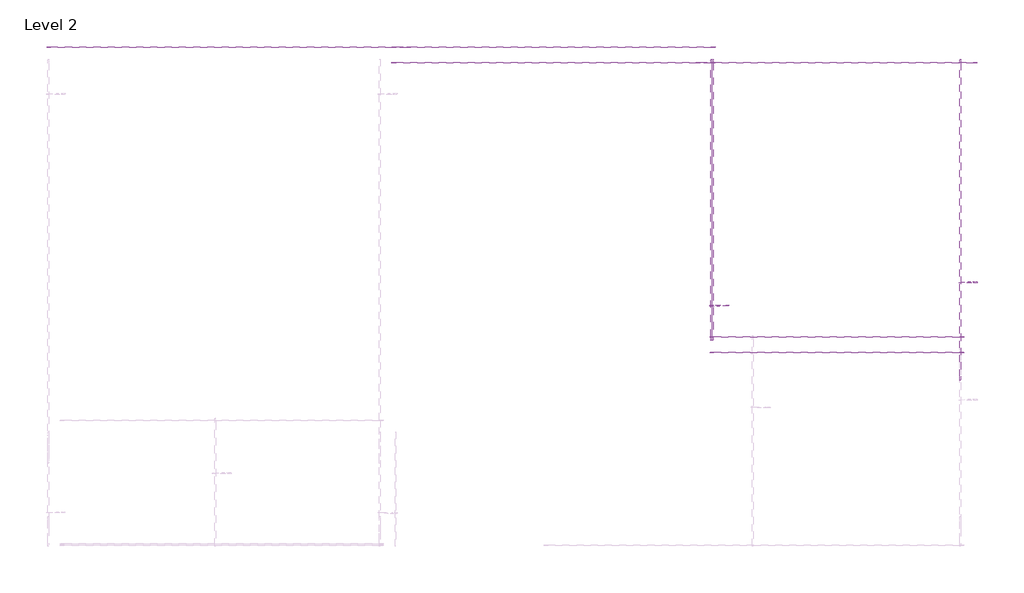
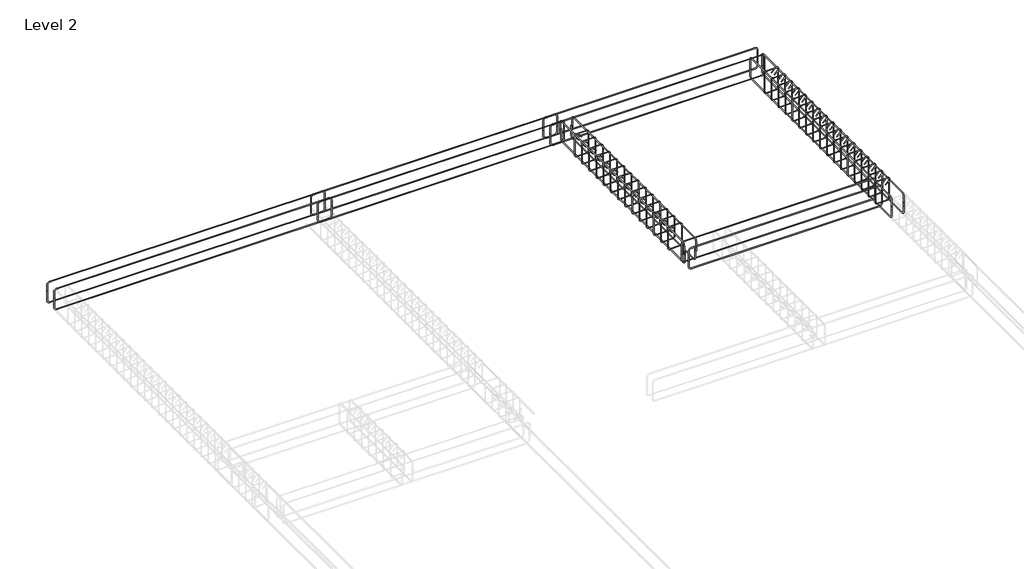
# One storey, part 5 of 5: 14 reinforcing bars.
"""IFC4 building model written with IfcOpenShell, lengths in millimetres."""

from ifc_helpers import new_model, si_unit, point, frame, origin, place, context, project, spatial, polyline, circle_curve, trimmed, segment, composite_curve, source, transform, mapped, element, save
from ifc_brep_helpers import swept_disk

model = new_model("IFC4")

# Units and contexts
model_context = context("Model", 3, world=origin())
ifc_project = project(units=[si_unit("LENGTHUNIT", "METRE", prefix="MILLI")], contexts=[model_context])

# Site, building, storey
site = spatial("IfcSite", under=ifc_project)
building = spatial("IfcBuilding", under=site)
storey = spatial("IfcBuildingStorey", under=building, Name="Level 2", Elevation=3048.0)

# Reinforcing bars
placement = place(None, origin())
reinforcing_bar_shape = source(origin(), model_context, "Body", "SolidModel", [
    swept_disk(composite_curve([segment(polyline([(-11033.7905379, 8472.592544, 5892.9032081), (-11033.7905379, 8472.592544, 5740.5032081)]), True, "CONTINUOUS"), segment(trimmed(circle_curve(frame((-11077.8595379, 8472.592544, 5740.5032081), z_axis=(0.0, 1.0, 0.0), x_axis=(44.068999999999505, 0.0, 0.0)), 44.069), [point((-11033.7905379, 8472.592544, 5740.5032081))], [point((-11077.8595379, 8472.592544, 5696.4342081))], True, "CARTESIAN"), True, "CONTINUOUS"), segment(polyline([(-11077.8595379, 8472.592544, 5696.4342081), (-15371.4835379, 8472.592544, 5696.4342081)]), True, "CONTINUOUS"), segment(trimmed(circle_curve(frame((-15371.4835379, 8472.592544, 5740.5032081), z_axis=(0.0, 1.0, 0.0), x_axis=(0.0, 0.0, -44.068999999999505)), 44.069), [point((-15371.4835379, 8472.592544, 5696.4342081))], [point((-15415.5525379, 8472.592544, 5740.5032081))], True, "CARTESIAN"), True, "CONTINUOUS"), segment(polyline([(-15415.5525379, 8472.592544, 5740.5032081), (-15415.5525379, 8472.592544, 5892.9032081)]), True, "CONTINUOUS")], self_intersect=False), 5.969),
])
element("IfcReinforcingBar", 1, at=placement, inside=storey, context=model_context, shape_type="MappedRepresentation", body=[
    mapped(reinforcing_bar_shape, transform((0.0, 0.0, 0.0), x_axis=(1.0, 0.0, 0.0), y_axis=(0.0, 1.0, 0.0), z_axis=(0.0, 0.0, 1.0))),
    mapped(reinforcing_bar_shape, transform((0.0, -189.5315837, 0.0), x_axis=(1.0, 0.0, 0.0), y_axis=(0.0, 1.0, 0.0), z_axis=(0.0, 0.0, 1.0))),
])
reinforcing_bar_2_shape = source(origin(), model_context, "Body", "SolidModel", [
    swept_disk(composite_curve([segment(polyline([(-15415.5525379, 8472.592544, 5841.8967919), (-15415.5525379, 8472.592544, 5994.2967919)]), True, "CONTINUOUS"), segment(trimmed(circle_curve(frame((-15371.4835379, 8472.592544, 5994.2967919), z_axis=(0.0, 1.0, 0.0), x_axis=(-44.068999999999505, 0.0, 0.0)), 44.069), [point((-15415.5525379, 8472.592544, 5994.2967919))], [point((-15371.4835379, 8472.592544, 6038.3657919))], True, "CARTESIAN"), True, "CONTINUOUS"), segment(polyline([(-15371.4835379, 8472.592544, 6038.3657919), (-11077.8595379, 8472.592544, 6038.3657919)]), True, "CONTINUOUS"), segment(trimmed(circle_curve(frame((-11077.8595379, 8472.592544, 5994.2967919), z_axis=(0.0, 1.0, 0.0), x_axis=(0.0, 0.0, 44.068999999999505)), 44.069), [point((-11077.8595379, 8472.592544, 6038.3657919))], [point((-11033.7905379, 8472.592544, 5994.2967919))], True, "CARTESIAN"), True, "CONTINUOUS"), segment(polyline([(-11033.7905379, 8472.592544, 5994.2967919), (-11033.7905379, 8472.592544, 5841.8967919)]), True, "CONTINUOUS")], self_intersect=False), 5.969),
])
element("IfcReinforcingBar", 2, at=placement, inside=storey, context=model_context, shape_type="MappedRepresentation", body=[
    mapped(reinforcing_bar_2_shape, transform((0.0, 0.0, 0.0), x_axis=(1.0, 0.0, 0.0), y_axis=(0.0, 1.0, 0.0), z_axis=(0.0, 0.0, 1.0))),
    mapped(reinforcing_bar_2_shape, transform((0.0, -189.5315837, 0.0), x_axis=(1.0, 0.0, 0.0), y_axis=(0.0, 1.0, 0.0), z_axis=(0.0, 0.0, 1.0))),
])
reinforcing_bar_3_shape = source(origin(), model_context, "Body", "SolidModel", [
    swept_disk(composite_curve([segment(polyline([(-11250.4525379, 8472.592544, 5841.8967919), (-11250.4525379, 8472.592544, 5994.2967919)]), True, "CONTINUOUS"), segment(trimmed(circle_curve(frame((-11206.3835379, 8472.592544, 5994.2967919), z_axis=(0.0, 1.0, 0.0), x_axis=(-44.069000000001324, 0.0, 0.0)), 44.069), [point((-11250.4525379, 8472.592544, 5994.2967919))], [point((-11206.3835379, 8472.592544, 6038.3657919))], True, "CARTESIAN"), True, "CONTINUOUS"), segment(polyline([(-11206.3835379, 8472.592544, 6038.3657919), (-7408.0595379, 8472.592544, 6038.3657919)]), True, "CONTINUOUS"), segment(trimmed(circle_curve(frame((-7408.0595379, 8472.592544, 5994.2967919), z_axis=(0.0, 1.0, 0.0), x_axis=(0.0, 0.0, 44.068999999999505)), 44.069), [point((-7408.0595379, 8472.592544, 6038.3657919))], [point((-7363.9905379, 8472.592544, 5994.2967919))], True, "CARTESIAN"), True, "CONTINUOUS"), segment(polyline([(-7363.9905379, 8472.592544, 5994.2967919), (-7363.9905379, 8472.592544, 5841.8967919)]), True, "CONTINUOUS")], self_intersect=False), 5.969),
])
element("IfcReinforcingBar", 3, at=placement, inside=storey, context=model_context, shape_type="MappedRepresentation", body=[
    mapped(reinforcing_bar_3_shape, transform((0.0, 0.0, 0.0), x_axis=(1.0, 0.0, 0.0), y_axis=(0.0, 1.0, 0.0), z_axis=(0.0, 0.0, 1.0))),
    mapped(reinforcing_bar_3_shape, transform((0.0, -189.5315837, 0.0), x_axis=(1.0, 0.0, 0.0), y_axis=(0.0, 1.0, 0.0), z_axis=(0.0, 0.0, 1.0))),
])
reinforcing_bar_4_shape = source(origin(), model_context, "Body", "SolidModel", [
    swept_disk(composite_curve([segment(polyline([(-7363.9905379, 8472.592544, 5892.9032081), (-7363.9905379, 8472.592544, 5740.5032081)]), True, "CONTINUOUS"), segment(trimmed(circle_curve(frame((-7408.0595379, 8472.592544, 5740.5032081), z_axis=(0.0, 1.0, 0.0), x_axis=(44.068999999999505, 0.0, 0.0)), 44.069), [point((-7363.9905379, 8472.592544, 5740.5032081))], [point((-7408.0595379, 8472.592544, 5696.4342081))], True, "CARTESIAN"), True, "CONTINUOUS"), segment(polyline([(-7408.0595379, 8472.592544, 5696.4342081), (-11206.3835379, 8472.592544, 5696.4342081)]), True, "CONTINUOUS"), segment(trimmed(circle_curve(frame((-11206.3835379, 8472.592544, 5740.5032081), z_axis=(0.0, 1.0, 0.0), x_axis=(0.0, 0.0, -44.068999999999505)), 44.069), [point((-11206.3835379, 8472.592544, 5696.4342081))], [point((-11250.4525379, 8472.592544, 5740.5032081))], True, "CARTESIAN"), True, "CONTINUOUS"), segment(polyline([(-11250.4525379, 8472.592544, 5740.5032081), (-11250.4525379, 8472.592544, 5892.9032081)]), True, "CONTINUOUS")], self_intersect=False), 5.969),
])
element("IfcReinforcingBar", 4, at=placement, inside=storey, context=model_context, shape_type="MappedRepresentation", body=[
    mapped(reinforcing_bar_4_shape, transform((0.0, 0.0, 0.0), x_axis=(1.0, 0.0, 0.0), y_axis=(0.0, 1.0, 0.0), z_axis=(0.0, 0.0, 1.0))),
    mapped(reinforcing_bar_4_shape, transform((0.0, -189.5315837, 0.0), x_axis=(1.0, 0.0, 0.0), y_axis=(0.0, 1.0, 0.0), z_axis=(0.0, 0.0, 1.0))),
])
reinforcing_bar_5_shape = source(origin(), model_context, "Body", "SolidModel", [
    swept_disk(composite_curve([segment(polyline([(-7580.6525379, 8472.592544, 5841.8967919), (-7580.6525379, 8472.592544, 5994.2967919)]), True, "CONTINUOUS"), segment(trimmed(circle_curve(frame((-7536.5835379, 8472.592544, 5994.2967919), z_axis=(0.0, 1.0, 0.0), x_axis=(-44.069000000000415, 0.0, 0.0)), 44.069), [point((-7580.6525379, 8472.592544, 5994.2967919))], [point((-7536.5835379, 8472.592544, 6038.3657919))], True, "CARTESIAN"), True, "CONTINUOUS"), segment(polyline([(-7536.5835379, 8472.592544, 6038.3657919), (-4242.9595379, 8472.592544, 6038.3657919)]), True, "CONTINUOUS"), segment(trimmed(circle_curve(frame((-4242.9595379, 8472.592544, 5994.2967919), z_axis=(0.0, 1.0, 0.0), x_axis=(0.0, 0.0, 44.068999999999505)), 44.069), [point((-4242.9595379, 8472.592544, 6038.3657919))], [point((-4198.8905379, 8472.592544, 5994.2967919))], True, "CARTESIAN"), True, "CONTINUOUS"), segment(polyline([(-4198.8905379, 8472.592544, 5994.2967919), (-4198.8905379, 8472.592544, 5841.8967919)]), True, "CONTINUOUS")], self_intersect=False), 5.969),
])
element("IfcReinforcingBar", 5, at=placement, inside=storey, context=model_context, shape_type="MappedRepresentation", body=[
    mapped(reinforcing_bar_5_shape, transform((0.0, 0.0, 0.0), x_axis=(1.0, 0.0, 0.0), y_axis=(0.0, 1.0, 0.0), z_axis=(0.0, 0.0, 1.0))),
    mapped(reinforcing_bar_5_shape, transform((0.0, -189.5315837, 0.0), x_axis=(1.0, 0.0, 0.0), y_axis=(0.0, 1.0, 0.0), z_axis=(0.0, 0.0, 1.0))),
])
reinforcing_bar_6_shape = source(origin(), model_context, "Body", "SolidModel", [
    swept_disk(composite_curve([segment(polyline([(-4198.8905379, 8472.592544, 5892.9032081), (-4198.8905379, 8472.592544, 5740.5032081)]), True, "CONTINUOUS"), segment(trimmed(circle_curve(frame((-4242.9595379, 8472.592544, 5740.5032081), z_axis=(0.0, 1.0, 0.0), x_axis=(44.069000000000415, 0.0, 0.0)), 44.069), [point((-4198.8905379, 8472.592544, 5740.5032081))], [point((-4242.9595379, 8472.592544, 5696.4342081))], True, "CARTESIAN"), True, "CONTINUOUS"), segment(polyline([(-4242.9595379, 8472.592544, 5696.4342081), (-7536.5835379, 8472.592544, 5696.4342081)]), True, "CONTINUOUS"), segment(trimmed(circle_curve(frame((-7536.5835379, 8472.592544, 5740.5032081), z_axis=(0.0, 1.0, 0.0), x_axis=(0.0, 0.0, -44.068999999999505)), 44.069), [point((-7536.5835379, 8472.592544, 5696.4342081))], [point((-7580.6525379, 8472.592544, 5740.5032081))], True, "CARTESIAN"), True, "CONTINUOUS"), segment(polyline([(-7580.6525379, 8472.592544, 5740.5032081), (-7580.6525379, 8472.592544, 5892.9032081)]), True, "CONTINUOUS")], self_intersect=False), 5.969),
])
element("IfcReinforcingBar", 6, at=placement, inside=storey, context=model_context, shape_type="MappedRepresentation", body=[
    mapped(reinforcing_bar_6_shape, transform((0.0, 0.0, 0.0), x_axis=(1.0, 0.0, 0.0), y_axis=(0.0, 1.0, 0.0), z_axis=(0.0, 0.0, 1.0))),
    mapped(reinforcing_bar_6_shape, transform((0.0, -189.5315837, 0.0), x_axis=(1.0, 0.0, 0.0), y_axis=(0.0, 1.0, 0.0), z_axis=(0.0, 0.0, 1.0))),
])
reinforcing_bar_7_shape = source(origin(), model_context, "Body", "SolidModel", [
    swept_disk(composite_curve([segment(polyline([(-4212.455746, 8321.0577522, 5841.8967919), (-4212.455746, 8321.0577522, 5994.2967919)]), True, "CONTINUOUS"), segment(trimmed(circle_curve(frame((-4212.455746, 8276.9887522, 5994.2967919), z_axis=(1.0, 0.0, 0.0), x_axis=(0.0, 44.068999999999505, 0.0)), 44.069), [point((-4212.455746, 8321.0577522, 5994.2967919))], [point((-4212.455746, 8276.9887522, 6038.3657919))], True, "CARTESIAN"), True, "CONTINUOUS"), segment(polyline([(-4212.455746, 8276.9887522, 6038.3657919), (-4212.455746, 4496.0647522, 6038.3657919)]), True, "CONTINUOUS"), segment(trimmed(circle_curve(frame((-4212.455746, 4496.0647522, 5994.2967919), z_axis=(1.0, 0.0, 0.0), x_axis=(0.0, 0.0, 44.068999999999505)), 44.069), [point((-4212.455746, 4496.0647522, 6038.3657919))], [point((-4212.455746, 4451.9957522, 5994.2967919))], True, "CARTESIAN"), True, "CONTINUOUS"), segment(polyline([(-4212.455746, 4451.9957522, 5994.2967919), (-4212.455746, 4451.9957522, 5841.8967919)]), True, "CONTINUOUS")], self_intersect=False), 5.969),
])
element("IfcReinforcingBar", 7, at=placement, inside=storey, context=model_context, shape_type="MappedRepresentation", body=[
    mapped(reinforcing_bar_7_shape, transform((0.0, 0.0, 0.0), x_axis=(1.0, 0.0, 0.0), y_axis=(0.0, 1.0, 0.0), z_axis=(0.0, 0.0, 1.0))),
    mapped(reinforcing_bar_7_shape, transform((-189.5315837, 0.0, 0.0), x_axis=(1.0, 0.0, 0.0), y_axis=(0.0, 1.0, 0.0), z_axis=(0.0, 0.0, 1.0))),
])
reinforcing_bar_8_shape = source(origin(), model_context, "Body", "SolidModel", [
    swept_disk(composite_curve([segment(polyline([(-4212.455746, 4451.9957522, 5892.9032081), (-4212.455746, 4451.9957522, 5740.5032081)]), True, "CONTINUOUS"), segment(trimmed(circle_curve(frame((-4212.455746, 4496.0647522, 5740.5032081), z_axis=(1.0, 0.0, 0.0), x_axis=(0.0, -44.068999999999505, 0.0)), 44.069), [point((-4212.455746, 4451.9957522, 5740.5032081))], [point((-4212.455746, 4496.0647522, 5696.4342081))], True, "CARTESIAN"), True, "CONTINUOUS"), segment(polyline([(-4212.455746, 4496.0647522, 5696.4342081), (-4212.455746, 8276.9887522, 5696.4342081)]), True, "CONTINUOUS"), segment(trimmed(circle_curve(frame((-4212.455746, 8276.9887522, 5740.5032081), z_axis=(1.0, 0.0, 0.0), x_axis=(0.0, 0.0, -44.068999999999505)), 44.069), [point((-4212.455746, 8276.9887522, 5696.4342081))], [point((-4212.455746, 8321.0577522, 5740.5032081))], True, "CARTESIAN"), True, "CONTINUOUS"), segment(polyline([(-4212.455746, 8321.0577522, 5740.5032081), (-4212.455746, 8321.0577522, 5892.9032081)]), True, "CONTINUOUS")], self_intersect=False), 5.969),
])
element("IfcReinforcingBar", 8, at=placement, inside=storey, context=model_context, shape_type="MappedRepresentation", body=[
    mapped(reinforcing_bar_8_shape, transform((0.0, 0.0, 0.0), x_axis=(1.0, 0.0, 0.0), y_axis=(0.0, 1.0, 0.0), z_axis=(0.0, 0.0, 1.0))),
    mapped(reinforcing_bar_8_shape, transform((-189.5315837, 0.0, 0.0), x_axis=(1.0, 0.0, 0.0), y_axis=(0.0, 1.0, 0.0), z_axis=(0.0, 0.0, 1.0))),
])
reinforcing_bar_9_shape = source(origin(), model_context, "Body", "SolidModel", [
    swept_disk(composite_curve([segment(polyline([(-4260.3161447, 7903.9897522, 5949.0166099), (-4205.4511463, 7903.9897522, 6003.8816084)]), True, "CONTINUOUS"), segment(trimmed(circle_curve(frame((-4226.1955379, 7903.9897522, 6024.626), z_axis=(0.0, -1.0, 0.0), x_axis=(20.7443916000002, 0.0, -20.7443916000002)), 29.337), [point((-4205.4511463, 7903.9897522, 6003.8816084))], [point((-4226.1955379, 7903.9897522, 6053.963))], True, "CARTESIAN"), True, "CONTINUOUS"), segment(polyline([(-4226.1955379, 7903.9897522, 6053.963), (-4388.2475379, 7903.9897522, 6053.963)]), True, "CONTINUOUS"), segment(trimmed(circle_curve(frame((-4388.2475379, 7903.9897522, 6024.626), z_axis=(0.0, -1.0, 0.0), x_axis=(0.0, 0.0, 29.336999999999534)), 29.337), [point((-4388.2475379, 7903.9897522, 6053.963))], [point((-4417.5845379, 7903.9897522, 6024.626))], True, "CARTESIAN"), True, "CONTINUOUS"), segment(polyline([(-4417.5845379, 7903.9897522, 6024.626), (-4417.5845379, 7903.9897522, 5710.174)]), True, "CONTINUOUS"), segment(trimmed(circle_curve(frame((-4388.2661869, 7905.0356312, 5710.174), z_axis=(0.03565051078635027, -0.9993643184948483, 0.0), x_axis=(-29.318350999999893, -1.045879000000241, 0.0)), 29.337), [point((-4417.5845379, 7903.9897522, 5710.174))], [point((-4388.2661869, 7905.0356312, 5680.837))], True, "CARTESIAN"), True, "CONTINUOUS"), segment(polyline([(-4388.2661869, 7905.0356312, 5680.837), (-4226.1768889, 7910.8178731, 5680.837)]), True, "CONTINUOUS"), segment(trimmed(circle_curve(frame((-4226.1768889, 7910.8178731, 5710.174), z_axis=(0.03565051078635027, -0.9993643184948483, 0.0), x_axis=(0.0, 0.0, -29.336999999999534)), 29.337), [point((-4226.1768889, 7910.8178731, 5680.837))], [point((-4196.8585379, 7911.8637522, 5710.174))], True, "CARTESIAN"), True, "CONTINUOUS"), segment(polyline([(-4196.8585379, 7911.8637522, 5710.174), (-4196.8585379, 7911.8637522, 6024.626)]), True, "CONTINUOUS"), segment(trimmed(circle_curve(frame((-4226.1955379, 7911.8637522, 6024.626), z_axis=(0.0, -1.0, 0.0), x_axis=(29.337000000000444, 0.0, 0.0)), 29.337), [point((-4196.8585379, 7911.8637522, 6024.626))], [point((-4246.9399295, 7911.8637522, 6045.3703916))], True, "CARTESIAN"), True, "CONTINUOUS"), segment(polyline([(-4246.9399295, 7911.8637522, 6045.3703916), (-4301.804928, 7911.8637522, 5990.5053932)]), True, "CONTINUOUS")], self_intersect=False), 3.937),
])
element("IfcReinforcingBar", 9, at=placement, inside=storey, context=model_context, shape_type="MappedRepresentation", body=[
    mapped(reinforcing_bar_9_shape, transform((0.0, 0.0, 0.0), x_axis=(1.0, 0.0, 0.0), y_axis=(0.0, 1.0, 0.0), z_axis=(0.0, 0.0, 1.0))),
    mapped(reinforcing_bar_9_shape, transform((0.0, -189.682875, 0.0), x_axis=(1.0, 0.0, 0.0), y_axis=(0.0, 1.0, 0.0), z_axis=(0.0, 0.0, 1.0))),
    mapped(reinforcing_bar_9_shape, transform((0.0, -379.36575, 0.0), x_axis=(1.0, 0.0, 0.0), y_axis=(0.0, 1.0, 0.0), z_axis=(0.0, 0.0, 1.0))),
    mapped(reinforcing_bar_9_shape, transform((0.0, -569.048625, 0.0), x_axis=(1.0, 0.0, 0.0), y_axis=(0.0, 1.0, 0.0), z_axis=(0.0, 0.0, 1.0))),
    mapped(reinforcing_bar_9_shape, transform((0.0, -758.7315, 0.0), x_axis=(1.0, 0.0, 0.0), y_axis=(0.0, 1.0, 0.0), z_axis=(0.0, 0.0, 1.0))),
    mapped(reinforcing_bar_9_shape, transform((0.0, -948.414375, 0.0), x_axis=(1.0, 0.0, 0.0), y_axis=(0.0, 1.0, 0.0), z_axis=(0.0, 0.0, 1.0))),
    mapped(reinforcing_bar_9_shape, transform((0.0, -1138.09725, 0.0), x_axis=(1.0, 0.0, 0.0), y_axis=(0.0, 1.0, 0.0), z_axis=(0.0, 0.0, 1.0))),
    mapped(reinforcing_bar_9_shape, transform((0.0, -1327.780125, 0.0), x_axis=(1.0, 0.0, 0.0), y_axis=(0.0, 1.0, 0.0), z_axis=(0.0, 0.0, 1.0))),
    mapped(reinforcing_bar_9_shape, transform((0.0, -1517.463, 0.0), x_axis=(1.0, 0.0, 0.0), y_axis=(0.0, 1.0, 0.0), z_axis=(0.0, 0.0, 1.0))),
    mapped(reinforcing_bar_9_shape, transform((0.0, -1707.145875, 0.0), x_axis=(1.0, 0.0, 0.0), y_axis=(0.0, 1.0, 0.0), z_axis=(0.0, 0.0, 1.0))),
    mapped(reinforcing_bar_9_shape, transform((0.0, -1896.82875, 0.0), x_axis=(1.0, 0.0, 0.0), y_axis=(0.0, 1.0, 0.0), z_axis=(0.0, 0.0, 1.0))),
    mapped(reinforcing_bar_9_shape, transform((0.0, -2086.511625, 0.0), x_axis=(1.0, 0.0, 0.0), y_axis=(0.0, 1.0, 0.0), z_axis=(0.0, 0.0, 1.0))),
    mapped(reinforcing_bar_9_shape, transform((0.0, -2276.1945, 0.0), x_axis=(1.0, 0.0, 0.0), y_axis=(0.0, 1.0, 0.0), z_axis=(0.0, 0.0, 1.0))),
    mapped(reinforcing_bar_9_shape, transform((0.0, -2465.877375, 0.0), x_axis=(1.0, 0.0, 0.0), y_axis=(0.0, 1.0, 0.0), z_axis=(0.0, 0.0, 1.0))),
    mapped(reinforcing_bar_9_shape, transform((0.0, -2655.56025, 0.0), x_axis=(1.0, 0.0, 0.0), y_axis=(0.0, 1.0, 0.0), z_axis=(0.0, 0.0, 1.0))),
    mapped(reinforcing_bar_9_shape, transform((0.0, -2845.243125, 0.0), x_axis=(1.0, 0.0, 0.0), y_axis=(0.0, 1.0, 0.0), z_axis=(0.0, 0.0, 1.0))),
    mapped(reinforcing_bar_9_shape, transform((0.0, -3034.926, 0.0), x_axis=(1.0, 0.0, 0.0), y_axis=(0.0, 1.0, 0.0), z_axis=(0.0, 0.0, 1.0))),
])
reinforcing_bar_10_shape = source(origin(), model_context, "Body", "SolidModel", [
    swept_disk(composite_curve([segment(polyline([(-7354.1269311, 5351.6637522, 5949.0166099), (-7408.9919295, 5351.6637522, 6003.8816084)]), True, "CONTINUOUS"), segment(trimmed(circle_curve(frame((-7388.2475379, 5351.6637522, 6024.626), z_axis=(0.0, 1.0, 0.0), x_axis=(-20.7443916000002, 0.0, -20.7443916000002)), 29.337), [point((-7408.9919295, 5351.6637522, 6003.8816084))], [point((-7388.2475379, 5351.6637522, 6053.963))], True, "CARTESIAN"), True, "CONTINUOUS"), segment(polyline([(-7388.2475379, 5351.6637522, 6053.963), (-7226.1955379, 5351.6637522, 6053.963)]), True, "CONTINUOUS"), segment(trimmed(circle_curve(frame((-7226.1955379, 5351.6637522, 6024.626), z_axis=(0.0, 1.0, 0.0), x_axis=(0.0, 0.0, 29.336999999999534)), 29.337), [point((-7226.1955379, 5351.6637522, 6053.963))], [point((-7196.8585379, 5351.6637522, 6024.626))], True, "CARTESIAN"), True, "CONTINUOUS"), segment(polyline([(-7196.8585379, 5351.6637522, 6024.626), (-7196.8585379, 5351.6637522, 5710.174)]), True, "CONTINUOUS"), segment(trimmed(circle_curve(frame((-7226.1768889, 5350.6178731, 5710.174), z_axis=(-0.03565051078635081, 0.9993643184948481, 0.0), x_axis=(29.318351000000803, 1.0458791000000929, 0.0)), 29.337), [point((-7196.8585379, 5351.6637522, 5710.174))], [point((-7226.1768889, 5350.6178731, 5680.837))], True, "CARTESIAN"), True, "CONTINUOUS"), segment(polyline([(-7226.1768889, 5350.6178731, 5680.837), (-7388.2661869, 5344.8356312, 5680.837)]), True, "CONTINUOUS"), segment(trimmed(circle_curve(frame((-7388.2661869, 5344.8356312, 5710.174), z_axis=(-0.03565051078635081, 0.9993643184948481, 0.0), x_axis=(0.0, 0.0, -29.336999999999534)), 29.337), [point((-7388.2661869, 5344.8356312, 5680.837))], [point((-7417.5845379, 5343.7897522, 5710.174))], True, "CARTESIAN"), True, "CONTINUOUS"), segment(polyline([(-7417.5845379, 5343.7897522, 5710.174), (-7417.5845379, 5343.7897522, 6024.626)]), True, "CONTINUOUS"), segment(trimmed(circle_curve(frame((-7388.2475379, 5343.7897522, 6024.626), z_axis=(0.0, 1.0, 0.0), x_axis=(-29.337000000000444, 0.0, 0.0)), 29.337), [point((-7417.5845379, 5343.7897522, 6024.626))], [point((-7367.5031463, 5343.7897522, 6045.3703916))], True, "CARTESIAN"), True, "CONTINUOUS"), segment(polyline([(-7367.5031463, 5343.7897522, 6045.3703916), (-7312.6381478, 5343.7897522, 5990.5053932)]), True, "CONTINUOUS")], self_intersect=False), 3.937),
])
element("IfcReinforcingBar", 10, at=placement, inside=storey, context=model_context, shape_type="MappedRepresentation", body=[
    mapped(reinforcing_bar_10_shape, transform((0.0, 0.0, 0.0), x_axis=(1.0, 0.0, 0.0), y_axis=(0.0, 1.0, 0.0), z_axis=(0.0, 0.0, 1.0))),
    mapped(reinforcing_bar_10_shape, transform((0.0, 196.3327692, 0.0), x_axis=(1.0, 0.0, 0.0), y_axis=(0.0, 1.0, 0.0), z_axis=(0.0, 0.0, 1.0))),
    mapped(reinforcing_bar_10_shape, transform((0.0, 392.6655385, 0.0), x_axis=(1.0, 0.0, 0.0), y_axis=(0.0, 1.0, 0.0), z_axis=(0.0, 0.0, 1.0))),
    mapped(reinforcing_bar_10_shape, transform((0.0, 588.9983077, 0.0), x_axis=(1.0, 0.0, 0.0), y_axis=(0.0, 1.0, 0.0), z_axis=(0.0, 0.0, 1.0))),
    mapped(reinforcing_bar_10_shape, transform((0.0, 785.3310769, 0.0), x_axis=(1.0, 0.0, 0.0), y_axis=(0.0, 1.0, 0.0), z_axis=(0.0, 0.0, 1.0))),
    mapped(reinforcing_bar_10_shape, transform((0.0, 981.6638462, 0.0), x_axis=(1.0, 0.0, 0.0), y_axis=(0.0, 1.0, 0.0), z_axis=(0.0, 0.0, 1.0))),
    mapped(reinforcing_bar_10_shape, transform((0.0, 1177.9966154, 0.0), x_axis=(1.0, 0.0, 0.0), y_axis=(0.0, 1.0, 0.0), z_axis=(0.0, 0.0, 1.0))),
    mapped(reinforcing_bar_10_shape, transform((0.0, 1374.3293846, 0.0), x_axis=(1.0, 0.0, 0.0), y_axis=(0.0, 1.0, 0.0), z_axis=(0.0, 0.0, 1.0))),
    mapped(reinforcing_bar_10_shape, transform((0.0, 1570.6621538, 0.0), x_axis=(1.0, 0.0, 0.0), y_axis=(0.0, 1.0, 0.0), z_axis=(0.0, 0.0, 1.0))),
    mapped(reinforcing_bar_10_shape, transform((0.0, 1766.9949231, 0.0), x_axis=(1.0, 0.0, 0.0), y_axis=(0.0, 1.0, 0.0), z_axis=(0.0, 0.0, 1.0))),
    mapped(reinforcing_bar_10_shape, transform((0.0, 1963.3276923, 0.0), x_axis=(1.0, 0.0, 0.0), y_axis=(0.0, 1.0, 0.0), z_axis=(0.0, 0.0, 1.0))),
    mapped(reinforcing_bar_10_shape, transform((0.0, 2159.6604615, 0.0), x_axis=(1.0, 0.0, 0.0), y_axis=(0.0, 1.0, 0.0), z_axis=(0.0, 0.0, 1.0))),
    mapped(reinforcing_bar_10_shape, transform((0.0, 2355.9932308, 0.0), x_axis=(1.0, 0.0, 0.0), y_axis=(0.0, 1.0, 0.0), z_axis=(0.0, 0.0, 1.0))),
    mapped(reinforcing_bar_10_shape, transform((0.0, 2552.326, 0.0), x_axis=(1.0, 0.0, 0.0), y_axis=(0.0, 1.0, 0.0), z_axis=(0.0, 0.0, 1.0))),
])
reinforcing_bar_11_shape = source(origin(), model_context, "Body", "SolidModel", [
    swept_disk(composite_curve([segment(polyline([(-7401.9873298, 4934.5957522, 5841.8967919), (-7401.9873298, 4934.5957522, 5994.2967919)]), True, "CONTINUOUS"), segment(trimmed(circle_curve(frame((-7401.9873298, 4978.6647522, 5994.2967919), z_axis=(-1.0, 0.0, 0.0), x_axis=(0.0, -44.069000000000415, 0.0)), 44.069), [point((-7401.9873298, 4934.5957522, 5994.2967919))], [point((-7401.9873298, 4978.6647522, 6038.3657919))], True, "CARTESIAN"), True, "CONTINUOUS"), segment(polyline([(-7401.9873298, 4978.6647522, 6038.3657919), (-7401.9873298, 8276.9887522, 6038.3657919)]), True, "CONTINUOUS"), segment(trimmed(circle_curve(frame((-7401.9873298, 8276.9887522, 5994.2967919), z_axis=(-1.0, 0.0, 0.0), x_axis=(0.0, 0.0, 44.068999999999505)), 44.069), [point((-7401.9873298, 8276.9887522, 6038.3657919))], [point((-7401.9873298, 8321.0577522, 5994.2967919))], True, "CARTESIAN"), True, "CONTINUOUS"), segment(polyline([(-7401.9873298, 8321.0577522, 5994.2967919), (-7401.9873298, 8321.0577522, 5841.8967919)]), True, "CONTINUOUS")], self_intersect=False), 5.969),
])
element("IfcReinforcingBar", 11, at=placement, inside=storey, context=model_context, shape_type="MappedRepresentation", body=[
    mapped(reinforcing_bar_11_shape, transform((0.0, 0.0, 0.0), x_axis=(1.0, 0.0, 0.0), y_axis=(0.0, 1.0, 0.0), z_axis=(0.0, 0.0, 1.0))),
    mapped(reinforcing_bar_11_shape, transform((189.5315837, 0.0, 0.0), x_axis=(1.0, 0.0, 0.0), y_axis=(0.0, 1.0, 0.0), z_axis=(0.0, 0.0, 1.0))),
])
reinforcing_bar_12_shape = source(origin(), model_context, "Body", "SolidModel", [
    swept_disk(composite_curve([segment(polyline([(-7226.1955379, 8321.0577522, 5887.212), (-7226.1955379, 8321.0577522, 5734.812)]), True, "CONTINUOUS"), segment(trimmed(circle_curve(frame((-7226.1955379, 8276.9887522, 5734.812), z_axis=(-1.0, 0.0, 0.0), x_axis=(0.0, 44.068999999999505, 0.0)), 44.069), [point((-7226.1955379, 8321.0577522, 5734.812))], [point((-7226.1955379, 8276.9887522, 5690.743))], True, "CARTESIAN"), True, "CONTINUOUS"), segment(polyline([(-7226.1955379, 8276.9887522, 5690.743), (-7226.1955379, 4978.6647522, 5690.743)]), True, "CONTINUOUS"), segment(trimmed(circle_curve(frame((-7226.1955379, 4978.6647522, 5734.812), z_axis=(-1.0, 0.0, 0.0), x_axis=(0.0, 0.0, -44.068999999999505)), 44.069), [point((-7226.1955379, 4978.6647522, 5690.743))], [point((-7226.1955379, 4934.5957522, 5734.812))], True, "CARTESIAN"), True, "CONTINUOUS"), segment(polyline([(-7226.1955379, 4934.5957522, 5734.812), (-7226.1955379, 4934.5957522, 5887.212)]), True, "CONTINUOUS")], self_intersect=False), 5.969),
])
element("IfcReinforcingBar", 12, at=placement, inside=storey, context=model_context, shape_type="MappedRepresentation", body=[
    mapped(reinforcing_bar_12_shape, transform((0.0, 0.0, 0.0), x_axis=(1.0, 0.0, 0.0), y_axis=(0.0, 1.0, 0.0), z_axis=(0.0, 0.0, 1.0))),
    mapped(reinforcing_bar_12_shape, transform((-162.052, 0.0, 0.0), x_axis=(1.0, 0.0, 0.0), y_axis=(0.0, 1.0, 0.0), z_axis=(0.0, 0.0, 1.0))),
])
reinforcing_bar_13_shape = source(origin(), model_context, "Body", "SolidModel", [
    swept_disk(composite_curve([segment(polyline([(-4363.9905379, 4783.0609603, 5841.8967919), (-4363.9905379, 4783.0609603, 5994.2967919)]), True, "CONTINUOUS"), segment(trimmed(circle_curve(frame((-4408.0595379, 4783.0609603, 5994.2967919), z_axis=(0.0, -1.0, 0.0), x_axis=(44.068999999999505, 0.0, 0.0)), 44.069), [point((-4363.9905379, 4783.0609603, 5994.2967919))], [point((-4408.0595379, 4783.0609603, 6038.3657919))], True, "CARTESIAN"), True, "CONTINUOUS"), segment(polyline([(-4408.0595379, 4783.0609603, 6038.3657919), (-7371.4835379, 4783.0609603, 6038.3657919)]), True, "CONTINUOUS"), segment(trimmed(circle_curve(frame((-7371.4835379, 4783.0609603, 5994.2967919), z_axis=(0.0, -1.0, 0.0), x_axis=(0.0, 0.0, 44.068999999999505)), 44.069), [point((-7371.4835379, 4783.0609603, 6038.3657919))], [point((-7415.5525379, 4783.0609603, 5994.2967919))], True, "CARTESIAN"), True, "CONTINUOUS"), segment(polyline([(-7415.5525379, 4783.0609603, 5994.2967919), (-7415.5525379, 4783.0609603, 5841.8967919)]), True, "CONTINUOUS")], self_intersect=False), 5.969),
])
element("IfcReinforcingBar", 13, at=placement, inside=storey, context=model_context, shape_type="MappedRepresentation", body=[
    mapped(reinforcing_bar_13_shape, transform((0.0, 0.0, 0.0), x_axis=(1.0, 0.0, 0.0), y_axis=(0.0, 1.0, 0.0), z_axis=(0.0, 0.0, 1.0))),
    mapped(reinforcing_bar_13_shape, transform((0.0, 189.5315837, 0.0), x_axis=(1.0, 0.0, 0.0), y_axis=(0.0, 1.0, 0.0), z_axis=(0.0, 0.0, 1.0))),
])
reinforcing_bar_14_shape = source(origin(), model_context, "Body", "SolidModel", [
    swept_disk(composite_curve([segment(polyline([(-7415.5525379, 4783.0609603, 5892.9032081), (-7415.5525379, 4783.0609603, 5740.5032081)]), True, "CONTINUOUS"), segment(trimmed(circle_curve(frame((-7371.4835379, 4783.0609603, 5740.5032081), z_axis=(0.0, -1.0, 0.0), x_axis=(-44.069000000000415, 0.0, 0.0)), 44.069), [point((-7415.5525379, 4783.0609603, 5740.5032081))], [point((-7371.4835379, 4783.0609603, 5696.4342081))], True, "CARTESIAN"), True, "CONTINUOUS"), segment(polyline([(-7371.4835379, 4783.0609603, 5696.4342081), (-4408.0595379, 4783.0609603, 5696.4342081)]), True, "CONTINUOUS"), segment(trimmed(circle_curve(frame((-4408.0595379, 4783.0609603, 5740.5032081), z_axis=(0.0, -1.0, 0.0), x_axis=(0.0, 0.0, -44.068999999999505)), 44.069), [point((-4408.0595379, 4783.0609603, 5696.4342081))], [point((-4363.9905379, 4783.0609603, 5740.5032081))], True, "CARTESIAN"), True, "CONTINUOUS"), segment(polyline([(-4363.9905379, 4783.0609603, 5740.5032081), (-4363.9905379, 4783.0609603, 5892.9032081)]), True, "CONTINUOUS")], self_intersect=False), 5.969),
])
element("IfcReinforcingBar", 14, at=placement, inside=storey, context=model_context, shape_type="MappedRepresentation", body=[
    mapped(reinforcing_bar_14_shape, transform((0.0, 0.0, 0.0), x_axis=(1.0, 0.0, 0.0), y_axis=(0.0, 1.0, 0.0), z_axis=(0.0, 0.0, 1.0))),
    mapped(reinforcing_bar_14_shape, transform((0.0, 189.5315837, 0.0), x_axis=(1.0, 0.0, 0.0), y_axis=(0.0, 1.0, 0.0), z_axis=(0.0, 0.0, 1.0))),
])

save(model, "model.ifc")

# Revit data of these elements
# Elements 1, 2, 3, 4, 5, 6, 7, 8, 9, 10, 11, 12, 13, 14 (IfcReinforcingBar)
#   Phase Created = New Construction
